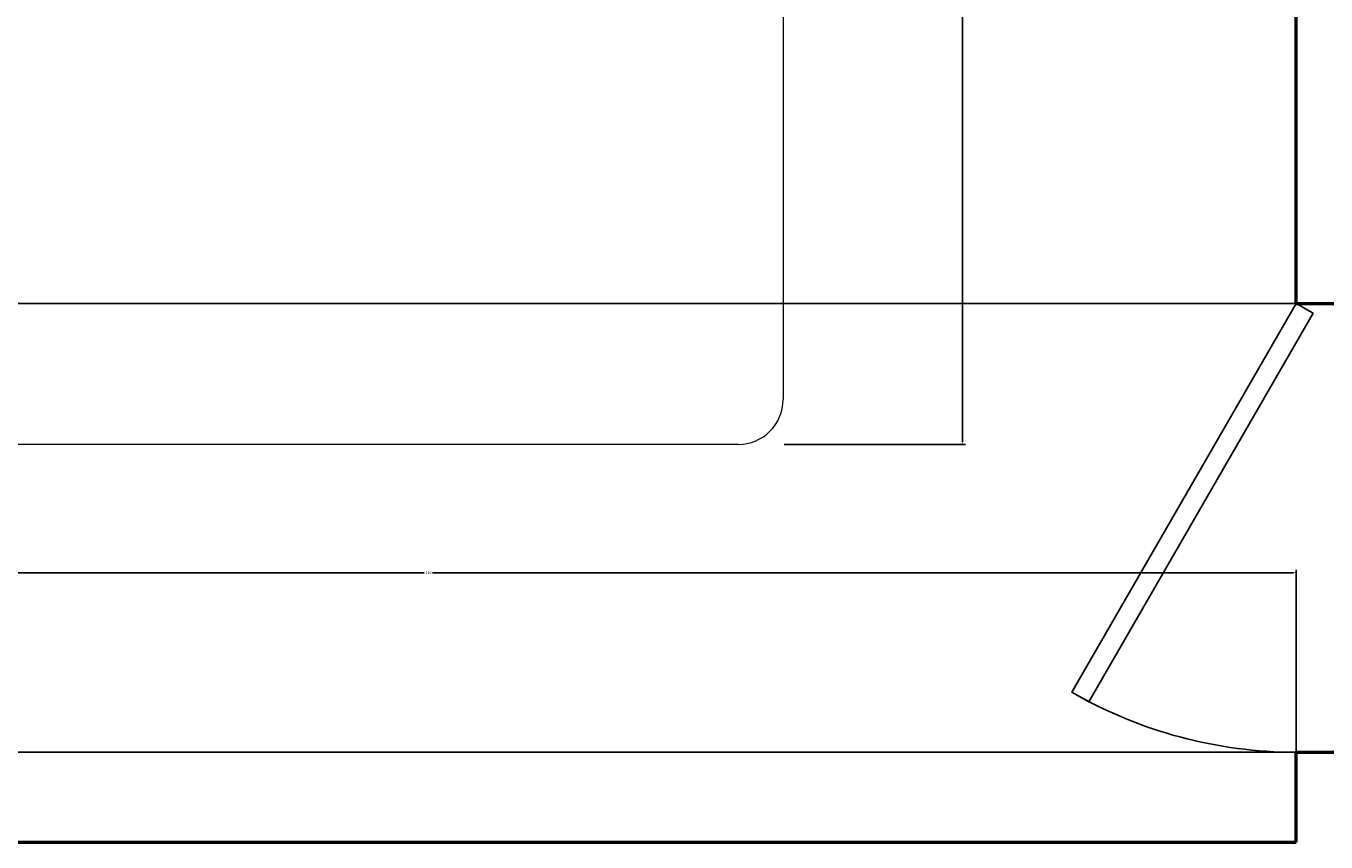
# Model space of a CAD drawing. Units: inches. Extents: x 2621 to 2849, y 2066 to 2463.
# Tile 16 of 28: x 2679 to 2766, y 2319 to 2374. Entities that reach past the tile are written whole.
import ezdxf

# ---------------------------------------------------------------- set-up
doc = ezdxf.new("R2010")
doc.units = ezdxf.units.IN
for name, color, linetype, lineweight in [('A-ANNO-DIMS', 2, 'Continuous', 18), ('A-DOOR', 3, 'Continuous', 25), ('A-FURN', 8, 'Continuous', 18), ('A-WALL', 7, 'Continuous', 50)]:
    doc.layers.add(name, color=color, linetype=linetype, lineweight=lineweight)
doc.styles.get("Standard").update_dxf_attribs({"font": 'arial.ttf'})
doc.dimstyles.get("Standard").update_dxf_attribs({"dimtxt": 0.18, "dimasz": 0.18, "dimexe": 0.18, "dimexo": 0.0625, "dimgap": 0.09, "dimtad": 0, "dimtih": 1, "dimtoh": 1, "dimdec": 4, "dimzin": 0, "dimdsep": 46, "dimtxsty": 'Standard', "dimcen": 0.09, "dimadec": 0, "dimazin": 0, "dimtfac": 1, "dimtdec": 4, "dimtofl": 0, "dimtmove": 0, "dimatfit": 3, "dimfxl": 1, "dimtolj": 1, "dimtzin": 0, "dimarcsym": 0})

# ---------------------------------------------------------------- blocks, each defined once
blk = doc.blocks.new('*U5')
for p, q in [((0, 0), (0, 6)), ((40, 0), (40, 6))]:
    blk.add_line(p, q)
blk.add_lwpolyline([(0, 0), (34.64, -20), (35.52, -18.48), (0.87, 1.52)], close=True)
blk.add_arc((0, 0), 40, 330, 0)
blk = doc.blocks.new('Bed - Queen')
for p, q in [((3, 0), (56.99999, 0)), ((10.99999, -1.2), (25.79998, -1.2)), ((34.19999, -1.2), (48.99999, -1.2)), ((0, -77.00003), (0, -3)), ((59.99999, -3), (59.99999, -77.00003)), ((7.99999, -14.4), (7.99999, -4.2)), ((28.79998, -4.2), (28.79998, -14.4)), ((31.19999, -14.4), (31.19999, -4.2)), ((51.99999, -4.2), (51.99999, -13.4)), ((0, -14.4), (44.8, -14.4)), ((59.99999, -29.6), (44.8, -14.4)), ((44.8, -14.4), (44.8, -26.6)), ((48.99999, -16.4), (46.79936, -16.4)), ((44.8, -16.8), (0, -16.8)), ((47.8, -29.6), (59.99999, -29.6)), ((56.99999, -80.00003), (3, -80.00003))]:
    blk.add_line(p, q)
for centre, start, end in [((3, -3), 90, 180), ((56.99999, -3), 0, 90), ((10.99999, -4.2), 90, 180), ((25.79998, -4.2), 0, 90), ((34.19999, -4.2), 90, 180), ((48.99999, -4.2), 0, 90), ((48.99999, -13.4), 270, 0), ((47.8, -26.6), 180, 270), ((3, -77.00003), 180, 270), ((56.99999, -77.00003), 270, 0)]:
    blk.add_arc(centre, 3, start, end)
blk = doc.blocks.new('*D16')
at = {"layer": 'A-ANNO-DIMS', "color": 0, "lineweight": -2, "transparency": 16777216}
for p, q in [((2729.644, 2405.954), (2741.761, 2405.954)), ((2741.581, 2405.774), (2741.581, 2376.136)), ((2741.581, 2346.134), (2741.581, 2375.772)), ((2729.644, 2345.954), (2741.761, 2345.954))]:
    blk.add_line(p, q, dxfattribs=at)
at = {"layer": 'A-ANNO-DIMS', "color": 0, "transparency": 16777216}
for points in [[(2741.551, 2405.774), (2741.611, 2405.774), (2741.581, 2405.954)], [(2741.551, 2346.134), (2741.611, 2346.134), (2741.581, 2345.954)]]:
    blk.add_solid(points, dxfattribs=at)
at = {"layer": 'Defpoints', "color": 0, "transparency": 16777216}
for p in [(2729.581, 2405.954), (2741.581, 2405.954), (2729.581, 2345.954)]:
    blk.add_point(p, dxfattribs=at)
at = {"layer": 'A-ANNO-DIMS', "color": 0, "transparency": 16777216, "insert": (2741.581, 2375.954), "char_height": 0.18, "attachment_point": 5}
blk.add_mtext('\\A1;60', dxfattribs=at)
blk = doc.blocks.new('*D45')
at = {"layer": 'A-ANNO-DIMS', "color": 0, "lineweight": -2, "transparency": 16777216}
for p, q in [((2647.87, 2319.437), (2647.87, 2337.558)), ((2648.05, 2337.378), (2705.59, 2337.378)), ((2763.69, 2337.378), (2706.15, 2337.378)), ((2763.87, 2319.437), (2763.87, 2337.558))]:
    blk.add_line(p, q, dxfattribs=at)
at = {"layer": 'A-ANNO-DIMS', "color": 0, "transparency": 16777216}
for points in [[(2648.05, 2337.408), (2648.05, 2337.348), (2647.87, 2337.378)], [(2763.69, 2337.408), (2763.69, 2337.348), (2763.87, 2337.378)]]:
    blk.add_solid(points, dxfattribs=at)
at = {"layer": 'Defpoints', "color": 0, "transparency": 16777216}
for p in [(2763.87, 2337.378), (2647.87, 2319.375), (2763.87, 2319.375)]:
    blk.add_point(p, dxfattribs=at)
at = {"layer": 'A-ANNO-DIMS', "color": 0, "transparency": 16777216, "insert": (2705.87, 2337.378), "char_height": 0.18, "attachment_point": 5}
blk.add_mtext('\\A1;116', dxfattribs=at)
blk = doc.blocks.new('*D50')
at = {"layer": 'A-ANNO-DIMS', "color": 0, "lineweight": -2, "transparency": 16777216}
for p, q in [((2763.808, 2355.375), (2620.687, 2355.375)), ((2620.867, 2355.195), (2620.867, 2340.557)), ((2620.867, 2325.555), (2620.867, 2340.193)), ((2763.808, 2325.375), (2620.687, 2325.375))]:
    blk.add_line(p, q, dxfattribs=at)
at = {"layer": 'A-ANNO-DIMS', "color": 0, "transparency": 16777216}
for points in [[(2620.837, 2355.195), (2620.897, 2355.195), (2620.867, 2355.375)], [(2620.837, 2325.555), (2620.897, 2325.555), (2620.867, 2325.375)]]:
    blk.add_solid(points, dxfattribs=at)
at = {"layer": 'Defpoints', "color": 0, "transparency": 16777216}
for p in [(2620.867, 2355.375), (2763.87, 2355.375), (2763.87, 2325.375)]:
    blk.add_point(p, dxfattribs=at)
at = {"layer": 'A-ANNO-DIMS', "color": 0, "transparency": 16777216, "insert": (2620.867, 2340.375), "char_height": 0.18, "attachment_point": 5}
blk.add_mtext('\\A1;30', dxfattribs=at)
blk = doc.blocks.new('*D51')
at = {"layer": 'A-ANNO-DIMS', "color": 0, "lineweight": -2, "transparency": 16777216}
for p, q in [((2763.808, 2325.375), (2620.687, 2325.375)), ((2620.867, 2325.195), (2620.867, 2322.556)), ((2620.867, 2319.555), (2620.867, 2322.193)), ((2763.808, 2319.375), (2620.687, 2319.375))]:
    blk.add_line(p, q, dxfattribs=at)
at = {"layer": 'A-ANNO-DIMS', "color": 0, "transparency": 16777216}
for points in [[(2620.837, 2325.195), (2620.897, 2325.195), (2620.867, 2325.375)], [(2620.837, 2319.555), (2620.897, 2319.555), (2620.867, 2319.375)]]:
    blk.add_solid(points, dxfattribs=at)
at = {"layer": 'Defpoints', "color": 0, "transparency": 16777216}
for p in [(2620.867, 2325.375), (2763.87, 2325.375), (2763.87, 2319.375)]:
    blk.add_point(p, dxfattribs=at)
at = {"layer": 'A-ANNO-DIMS', "color": 0, "transparency": 16777216, "insert": (2620.867, 2322.375), "char_height": 0.18, "attachment_point": 5}
blk.add_mtext('\\A1;6', dxfattribs=at)

msp = doc.modelspace()

# ---------------------------------------------------------------- linework, layer by layer
at = {"layer": 'A-WALL'}
for p, q in [((2763.8701, 2355.3746), (2763.8701, 2435.3746)), ((2763.8701, 2355.3746), (2767.8701, 2355.3746)), ((2763.8701, 2319.3746), (2763.8701, 2325.3746)), ((2763.8701, 2325.3746), (2767.8701, 2325.3746)), ((2647.8701, 2319.3746), (2763.8701, 2319.3746))]:
    msp.add_line(p, q, dxfattribs=at)

# ---------------------------------------------------------------- block references
at = {"layer": 'A-DOOR', "xscale": 0.75, "yscale": 0.75, "zscale": 0.75, "rotation": 270}
msp.add_blockref('*U5', (2763.8701, 2355.3746), dxfattribs=at)
at = {"layer": 'A-FURN', "rotation": 90}
msp.add_blockref('Bed - Queen', (2649.5811, 2345.9537), dxfattribs=at)

# ---------------------------------------------------------------- dimensions: what is measured, and where the dimension line sits
at = {"layer": 'A-ANNO-DIMS'}
for base, p1, p2, picture, middle in [((2741.5811, 2405.9537), (2729.5811, 2345.9537), (2729.5811, 2405.9537), '*D16', (2741.5811, 2375.9537)), ((2620.8666, 2355.3746), (2763.8701, 2325.3746), (2763.8701, 2355.3746), '*D50', (2620.8666, 2340.3746)), ((2620.8666, 2325.3746), (2763.8701, 2319.3746), (2763.8701, 2325.3746), '*D51', (2620.8666, 2322.3746))]:
    dim = msp.add_linear_dim(base=base, p1=p1, p2=p2, angle=90, dimstyle='Standard', override={"dimdec": 0, "dimlfac": 1, "dimrnd": 0, "dimzin": 0, "dimdsep": 46, "dimlunit": 2}, dxfattribs=at)
    dim.commit()
    dim.dimension.update_dxf_attribs({"geometry": picture, "text_midpoint": middle})
dim = msp.add_linear_dim(base=(2763.8701, 2337.3781), p1=(2647.8701, 2319.3746), p2=(2763.8701, 2319.3746), dimstyle='Standard', override={"dimdec": 0, "dimlfac": 1, "dimrnd": 0, "dimzin": 0, "dimdsep": 46, "dimlunit": 2}, dxfattribs=at)
dim.commit()
dim.dimension.update_dxf_attribs({"geometry": '*D45', "text_midpoint": (2705.8701, 2337.3781)})

doc.saveas('drawing.dxf')
